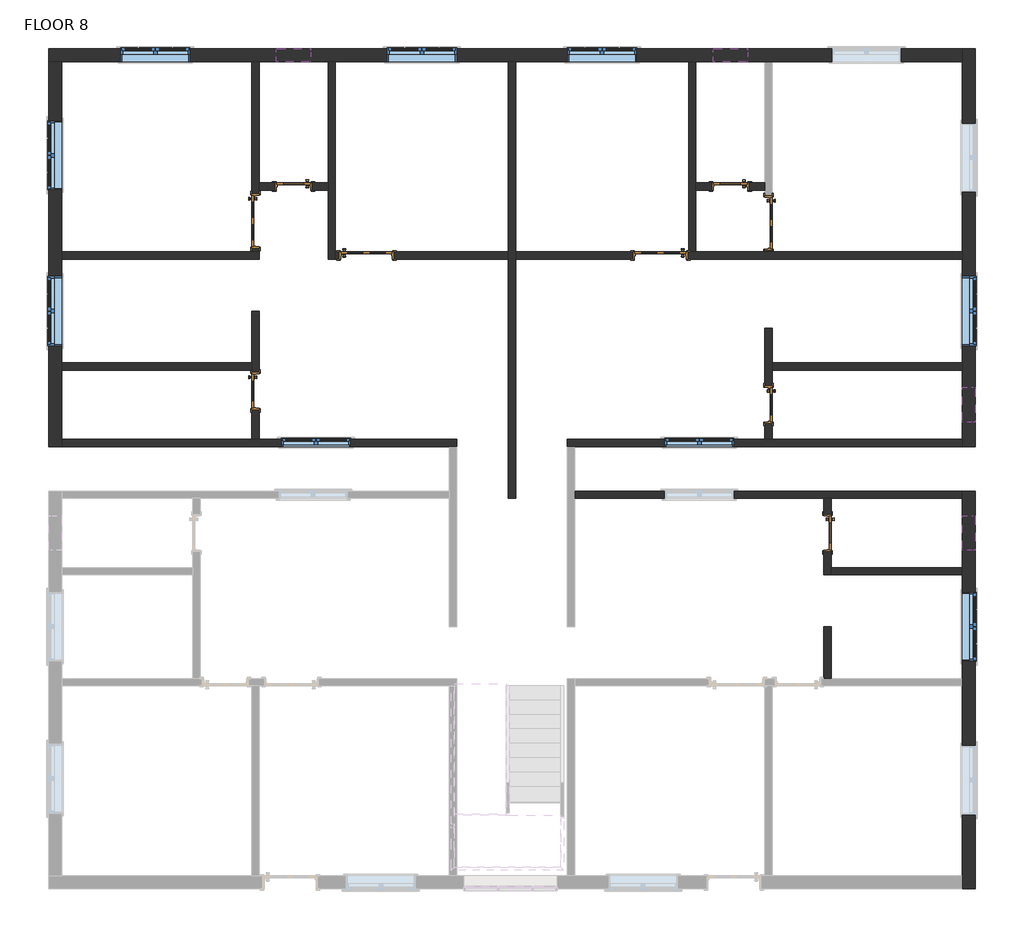
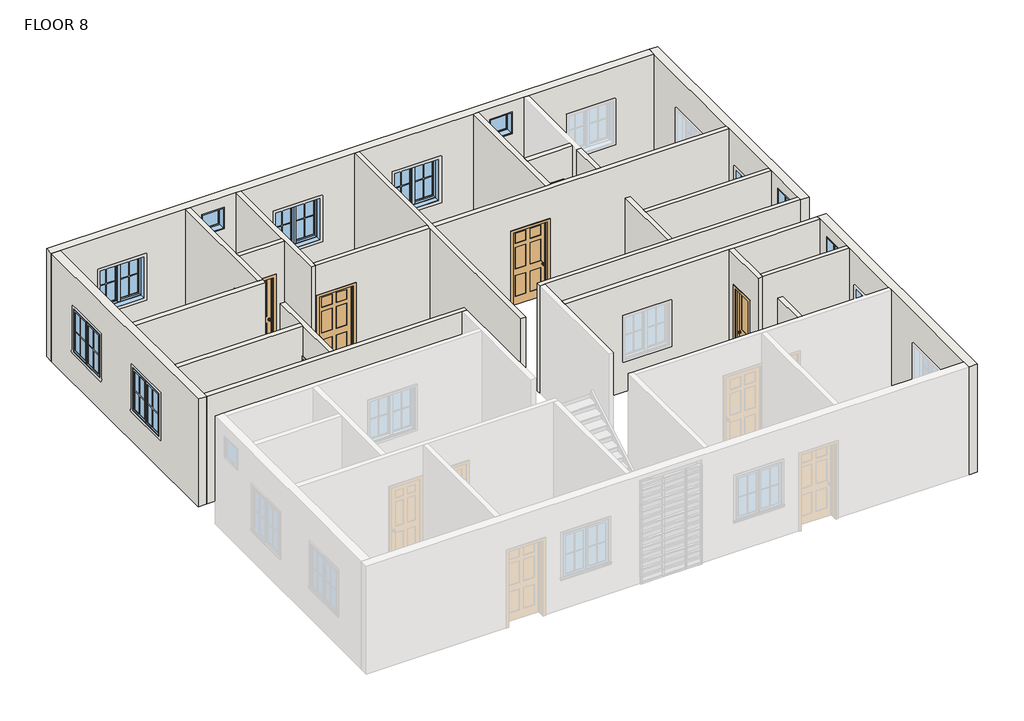
# One storey, part 3 of 4: 24 walls, 13 windows, 9 doors.
"""IFC4 building model written with IfcOpenShell, lengths in millimetres."""

from ifc_helpers import new_model, si_unit, frame, origin, place, context, project, spatial, polyline, outline, extrude, faceted_brep, transform, mapped, element, save
from components import door_e337afa5, door_596d7c92, door_c610b25b, door_03e3dfb5, window_80340324, window_9200f5ac, window_c2c97eee

model = new_model("IFC4")

# Units and contexts
model_context = context("Model", 3, world=origin())
ifc_project = project(units=[si_unit("LENGTHUNIT", "METRE", prefix="MILLI")], contexts=[model_context])

# Site, building, storey
site = spatial("IfcSite", under=ifc_project)
building = spatial("IfcBuilding", under=site)
storey = spatial("IfcBuildingStorey", under=building, Name="FLOOR 8", Elevation=12744.7725604)

# Doors
placement = place(None, origin())
door_shape = door_e337afa5(model_context)
element("IfcDoor", 1, ObjectType="Door-Interior-Single-2_Panel-Wood : 24\" x 84\"", at=placement, inside=storey, context=model_context, shape_type="MappedRepresentation", body=[
    mapped(door_shape, transform((-8112.4137331, 4563.2156164, 12744.7725604), x_axis=(-1.0, 0.0, 0.0), y_axis=(0.0, -1.0, 0.0), z_axis=(0.0, 0.0, 1.0))),
])
element("IfcDoor", 2, ObjectType="Door-Interior-Single-2_Panel-Wood : 24\" x 84\"", at=placement, inside=storey, context=model_context, shape_type="MappedRepresentation", body=[
    mapped(door_shape, transform((-416.2137331, 4563.2156164, 12744.7725604), x_axis=(-1.0, 0.0, 0.0), y_axis=(0.0, -1.0, 0.0), z_axis=(0.0, 0.0, 1.0))),
])
element("IfcDoor", 3, ObjectType="Door-Interior-Single-2_Panel-Wood : 24\" x 84\"", at=placement, inside=storey, context=model_context, shape_type="MappedRepresentation", body=[
    mapped(door_shape, transform((-8788.6887331, 953.2406164, 12744.7725604), x_axis=(0.0, -1.0, 0.0), y_axis=(1.0, 0.0, 0.0), z_axis=(0.0, 0.0, 1.0))),
])
door_2_shape = door_596d7c92(model_context)
element("IfcDoor", 4, ObjectType="Door-Interior-Single-2_Panel-Wood : 24\" x 84\"", at=placement, inside=storey, context=model_context, shape_type="MappedRepresentation", body=[
    mapped(door_2_shape, transform((260.0612669, 711.9406164, 12744.7725604), x_axis=(0.0, -1.0, 0.0), y_axis=(1.0, 0.0, 0.0), z_axis=(0.0, 0.0, 1.0))),
])
element("IfcDoor", 5, ObjectType="Door-Interior-Single-2_Panel-Wood : 24\" x 84\"", at=placement, inside=storey, context=model_context, shape_type="MappedRepresentation", body=[
    mapped(door_2_shape, transform((1301.4612669, -1548.6593836, 12744.7725604), x_axis=(0.0, -1.0, 0.0), y_axis=(1.0, 0.0, 0.0), z_axis=(0.0, 0.0, 1.0))),
])
door_3_shape = door_c610b25b(model_context)
element("IfcDoor", 6, ObjectType="Door-Interior-Single-6_Panel-Wood : 36\" x 84\"", at=placement, inside=storey, context=model_context, shape_type="MappedRepresentation", body=[
    mapped(door_3_shape, transform((-8788.6887331, 3950.4406164, 12744.7725604), x_axis=(0.0, -1.0, 0.0), y_axis=(1.0, 0.0, 0.0), z_axis=(0.0, 0.0, 1.0))),
])
element("IfcDoor", 7, ObjectType="Door-Interior-Single-6_Panel-Wood : 36\" x 84\"", at=placement, inside=storey, context=model_context, shape_type="MappedRepresentation", body=[
    mapped(door_3_shape, transform((-1648.1137331, 3344.0156164, 12744.7725604), x_axis=(-1.0, 0.0, 0.0), y_axis=(0.0, -1.0, 0.0), z_axis=(0.0, 0.0, 1.0))),
])
door_4_shape = door_03e3dfb5(model_context)
element("IfcDoor", 8, ObjectType="Door-Interior-Single-6_Panel-Wood : 36\" x 84\"", at=placement, inside=storey, context=model_context, shape_type="MappedRepresentation", body=[
    mapped(door_4_shape, transform((-6829.7137331, 3344.0156164, 12744.7725604), x_axis=(1.0, 0.0, 0.0), y_axis=(0.0, 1.0, 0.0), z_axis=(0.0, 0.0, 1.0))),
])
element("IfcDoor", 9, ObjectType="Door-Interior-Single-6_Panel-Wood : 36\" x 84\"", at=placement, inside=storey, context=model_context, shape_type="MappedRepresentation", body=[
    mapped(door_4_shape, transform((260.0612669, 3912.3406164, 12744.7725604), x_axis=(0.0, -1.0, 0.0), y_axis=(1.0, 0.0, 0.0), z_axis=(0.0, 0.0, 1.0))),
])

# Walls
element("IfcWall", 10, ObjectType="Inner Wall 5\"", at=placement, inside=storey, context=model_context, shape_type="Brep", body=[
    faceted_brep([(-12201.8137331, -24.6593836, 12744.7725604), (-5369.2137331, -24.6593836, 12744.7725604), (-5242.2137331, -24.6593836, 12744.7725604), (-5242.2137331, -24.6593836, 15792.7725604), (-5369.2137331, -24.6593836, 15792.7725604), (-12201.8137331, -24.6593836, 15792.7725604), (-7109.1137331, -24.6593836, 14878.3725604), (-7109.1137331, -24.6593836, 13659.1725604), (-8328.3137331, -24.6593836, 13659.1725604), (-8328.3137331, -24.6593836, 14878.3725604), (-12201.8137331, 102.3406164, 12744.7725604), (-12201.8137331, 102.3406164, 15792.7725604), (-8849.0137331, 102.3406164, 15792.7725604), (-8722.0137331, 102.3406164, 15792.7725604), (-5242.2137331, 102.3406164, 15792.7725604), (-5242.2137331, 102.3406164, 12744.7725604), (-8722.0137331, 102.3406164, 12744.7725604), (-8849.0137331, 102.3406164, 12744.7725604), (-7109.1137331, 102.3406164, 14878.3725604), (-8328.3137331, 102.3406164, 14878.3725604), (-8328.3137331, 102.3406164, 13659.1725604), (-7109.1137331, 102.3406164, 13659.1725604)], [[[0, 1, 2, 3, 4, 5], [6, 7, 8, 9]], [[10, 11, 12, 13, 14, 15, 16, 17], [18, 19, 20, 21]], [[2, 1, 0, 10, 17, 16, 15]], [[5, 4, 3, 14, 13, 12, 11]], [[0, 5, 11, 10]], [[3, 2, 15, 14]], [[7, 6, 18, 21]], [[8, 7, 21, 20]], [[9, 8, 20, 19]], [[6, 9, 19, 18]]]),
])
element("IfcWall", 11, ObjectType="Inner Wall 5\"", at=placement, inside=storey, context=model_context, shape_type="Brep", body=[
    faceted_brep([(3673.1862669, 102.3406164, 12744.7725604), (320.3862669, 102.3406164, 12744.7725604), (193.3862669, 102.3406164, 12744.7725604), (-3286.4137331, 102.3406164, 12744.7725604), (-3286.4137331, 102.3406164, 15792.7725604), (193.3862669, 102.3406164, 15792.7725604), (320.3862669, 102.3406164, 15792.7725604), (3673.1862669, 102.3406164, 15792.7725604), (-352.7137331, 102.3406164, 14878.3725604), (-1571.9137331, 102.3406164, 14878.3725604), (-1571.9137331, 102.3406164, 13659.1725604), (-352.7137331, 102.3406164, 13659.1725604), (3673.1862669, -24.6593836, 12744.7725604), (3673.1862669, -24.6593836, 15792.7725604), (-3159.4137331, -24.6593836, 15792.7725604), (-3286.4137331, -24.6593836, 15792.7725604), (-3286.4137331, -24.6593836, 12744.7725604), (-3159.4137331, -24.6593836, 12744.7725604), (-352.7137331, -24.6593836, 14878.3725604), (-352.7137331, -24.6593836, 13659.1725604), (-1571.9137331, -24.6593836, 13659.1725604), (-1571.9137331, -24.6593836, 14878.3725604)], [[[0, 1, 2, 3, 4, 5, 6, 7], [8, 9, 10, 11]], [[12, 13, 14, 15, 16, 17], [18, 19, 20, 21]], [[3, 2, 1, 0, 12, 17, 16]], [[7, 6, 5, 4, 15, 14, 13]], [[0, 7, 13, 12]], [[4, 3, 16, 15]], [[19, 18, 8, 11]], [[20, 19, 11, 10]], [[21, 20, 10, 9]], [[18, 21, 9, 8]]]),
])
element("IfcWall", 12, ObjectType="Inner Wall 5\"", at=placement, inside=storey, context=model_context, shape_type="Brep", body=[
    faceted_brep([(3673.1862669, -812.0593836, 12744.7725604), (-3159.4137331, -812.0593836, 12744.7725604), (-3159.4137331, -812.0593836, 15792.7725604), (3673.1862669, -812.0593836, 15792.7725604), (-352.7137331, -812.0593836, 14878.3725604), (-1571.9137331, -812.0593836, 14878.3725604), (-1571.9137331, -812.0593836, 13659.1725604), (-352.7137331, -812.0593836, 13659.1725604), (3673.1862669, -939.0593836, 12744.7725604), (3673.1862669, -939.0593836, 15792.7725604), (1361.7862669, -939.0593836, 15792.7725604), (1234.7862669, -939.0593836, 15792.7725604), (-3159.4137331, -939.0593836, 15792.7725604), (-3159.4137331, -939.0593836, 12744.7725604), (1234.7862669, -939.0593836, 12744.7725604), (1361.7862669, -939.0593836, 12744.7725604), (-352.7137331, -939.0593836, 14878.3725604), (-352.7137331, -939.0593836, 13659.1725604), (-1571.9137331, -939.0593836, 13659.1725604), (-1571.9137331, -939.0593836, 14878.3725604)], [[[0, 1, 2, 3], [4, 5, 6, 7]], [[8, 9, 10, 11, 12, 13, 14, 15], [16, 17, 18, 19]], [[1, 0, 8, 15, 14, 13]], [[3, 2, 12, 11, 10, 9]], [[0, 3, 9, 8]], [[2, 1, 13, 12]], [[17, 16, 4, 7]], [[18, 17, 7, 6]], [[19, 18, 6, 5]], [[16, 19, 5, 4]]]),
])
element("IfcWall", 13, ObjectType="Inner Wall 5\"", at=placement, inside=storey, context=model_context, shape_type="Brep", body=[
    faceted_brep([(1234.7862669, -2285.2593836, 15792.7725604), (1234.7862669, -939.0593836, 15792.7725604), (1234.7862669, -939.0593836, 12744.7725604), (1234.7862669, -1218.4593836, 12744.7725604), (1234.7862669, -1218.4593836, 14903.7725604), (1234.7862669, -1878.8593836, 14903.7725604), (1234.7862669, -1878.8593836, 12744.7725604), (1234.7862669, -2285.2593836, 12744.7725604), (1361.7862669, -939.0593836, 15792.7725604), (1361.7862669, -2158.2593836, 15792.7725604), (1361.7862669, -2285.2593836, 15792.7725604), (1361.7862669, -2285.2593836, 12744.7725604), (1361.7862669, -2158.2593836, 12744.7725604), (1361.7862669, -1878.8593836, 12744.7725604), (1361.7862669, -1878.8593836, 14903.7725604), (1361.7862669, -1218.4593836, 14903.7725604), (1361.7862669, -1218.4593836, 12744.7725604), (1361.7862669, -939.0593836, 12744.7725604)], [[[0, 1, 2, 3, 4, 5, 6, 7]], [[8, 9, 10, 11, 12, 13, 14, 15, 16, 17]], [[2, 17, 16, 3]], [[11, 7, 6, 13, 12]], [[1, 0, 10, 9, 8]], [[2, 1, 8, 17]], [[0, 7, 11, 10]], [[5, 14, 13, 6]], [[14, 5, 4, 15]], [[15, 4, 3, 16]]]),
])
element("IfcWall", 14, ObjectType="Inner Wall 5\"", at=placement, inside=storey, context=model_context, shape_type="SweptSolid", body=[
    extrude(outline(polyline([(3673.1862669, -2285.2593836), (1361.7862669, -2285.2593836), (1361.7862669, -2158.2593836), (3673.1862669, -2158.2593836), (3673.1862669, -2285.2593836)])), frame((0.0, 0.0, 12744.7725604), z_axis=(0.0, 0.0, 1.0), x_axis=(1.0, 0.0, 0.0)), (0.0, 0.0, 1.0), 3048.0),
])
element("IfcWall", 15, ObjectType="Inner Wall 5\"", at=placement, inside=storey, context=model_context, shape_type="SweptSolid", body=[
    extrude(outline(polyline([(1361.7862669, -3199.6593836), (1361.7862669, -4114.0593836), (1234.7862669, -4114.0593836), (1234.7862669, -3199.6593836), (1361.7862669, -3199.6593836)])), frame((0.0, 0.0, 12744.7725604), z_axis=(0.0, 0.0, 1.0), x_axis=(1.0, 0.0, 0.0)), (0.0, 0.0, 1.0), 3048.0),
])
element("IfcWall", 16, ObjectType="Inner Wall 5\"", at=placement, inside=storey, context=model_context, shape_type="Brep", body=[
    faceted_brep([(-12201.8137331, 3277.3406164, 12744.7725604), (-8722.0137331, 3277.3406164, 12744.7725604), (-8722.0137331, 3277.3406164, 15792.7725604), (-12201.8137331, 3277.3406164, 15792.7725604), (-12201.8137331, 3404.3406164, 12744.7725604), (-12201.8137331, 3404.3406164, 15792.7725604), (-8849.0137331, 3404.3406164, 15792.7725604), (-8722.0137331, 3404.3406164, 15792.7725604), (-8722.0137331, 3404.3406164, 12744.7725604), (-8849.0137331, 3404.3406164, 12744.7725604)], [[[0, 1, 2, 3]], [[4, 5, 6, 7, 8, 9]], [[1, 0, 4, 9, 8]], [[3, 2, 7, 6, 5]], [[0, 3, 5, 4]], [[2, 1, 8, 7]]]),
])
element("IfcWall", 17, ObjectType="Inner Wall 5\"", at=placement, inside=storey, context=model_context, shape_type="Brep", body=[
    faceted_brep([(-8722.0137331, 6758.7281164, 15792.7725604), (-8722.0137331, 4623.5406164, 15792.7725604), (-8722.0137331, 4496.5406164, 15792.7725604), (-8722.0137331, 3404.3406164, 15792.7725604), (-8722.0137331, 3404.3406164, 12744.7725604), (-8722.0137331, 3467.8406164, 12744.7725604), (-8722.0137331, 3467.8406164, 14903.7725604), (-8722.0137331, 4433.0406164, 14903.7725604), (-8722.0137331, 4433.0406164, 12744.7725604), (-8722.0137331, 4496.5406164, 12744.7725604), (-8722.0137331, 4623.5406164, 12744.7725604), (-8722.0137331, 6758.7281164, 12744.7725604), (-8849.0137331, 3404.3406164, 15792.7725604), (-8849.0137331, 6758.7281164, 15792.7725604), (-8849.0137331, 6758.7281164, 12744.7725604), (-8849.0137331, 4433.0406164, 12744.7725604), (-8849.0137331, 4433.0406164, 14903.7725604), (-8849.0137331, 3467.8406164, 14903.7725604), (-8849.0137331, 3467.8406164, 12744.7725604), (-8849.0137331, 3404.3406164, 12744.7725604)], [[[0, 1, 2, 3, 4, 5, 6, 7, 8, 9, 10, 11]], [[12, 13, 14, 15, 16, 17, 18, 19]], [[4, 19, 18, 5]], [[14, 11, 10, 9, 8, 15]], [[3, 2, 1, 0, 13, 12]], [[4, 3, 12, 19]], [[0, 11, 14, 13]], [[17, 6, 5, 18]], [[6, 17, 16, 7]], [[7, 16, 15, 8]]]),
])
element("IfcWall", 18, ObjectType="Inner Wall 5\"", at=placement, inside=storey, context=model_context, shape_type="SweptSolid", body=[
    extrude(outline(polyline([(15792.7725604, -7502.8137331), (15792.7725604, -8722.0137331), (12744.7725604, -8722.0137331), (12744.7725604, -8442.6137331), (14903.7725604, -8442.6137331), (14903.7725604, -7782.2137331), (12744.7725604, -7782.2137331), (12744.7725604, -7502.8137331), (15792.7725604, -7502.8137331)])), frame((0.0, 4496.5406164, 0.0), z_axis=(0.0, 1.0, 0.0), x_axis=(0.0, 0.0, 1.0)), (0.0, 0.0, 1.0), 127.0),
])
element("IfcWall", 19, ObjectType="Inner Wall 5\"", at=placement, inside=storey, context=model_context, shape_type="Brep", body=[
    faceted_brep([(-7375.8137331, 3277.3406164, 12744.7725604), (-7375.8137331, 3404.3406164, 12744.7725604), (-7375.8137331, 6758.7281164, 12744.7725604), (-7375.8137331, 6758.7281164, 15792.7725604), (-7375.8137331, 3404.3406164, 15792.7725604), (-7375.8137331, 3277.3406164, 15792.7725604), (-7502.8137331, 3277.3406164, 12744.7725604), (-7502.8137331, 3277.3406164, 15792.7725604), (-7502.8137331, 4496.5406164, 15792.7725604), (-7502.8137331, 4623.5406164, 15792.7725604), (-7502.8137331, 6758.7281164, 15792.7725604), (-7502.8137331, 6758.7281164, 12744.7725604), (-7502.8137331, 4623.5406164, 12744.7725604), (-7502.8137331, 4496.5406164, 12744.7725604)], [[[0, 1, 2, 3, 4, 5]], [[6, 7, 8, 9, 10, 11, 12, 13]], [[2, 1, 0, 6, 13, 12, 11]], [[5, 4, 3, 10, 9, 8, 7]], [[3, 2, 11, 10]], [[0, 5, 7, 6]]]),
])
element("IfcWall", 20, ObjectType="Inner Wall 5\"", at=placement, inside=storey, context=model_context, shape_type="Brep", body=[
    faceted_brep([(-4327.8137331, 6758.7281164, 12744.7725604), (-4327.8137331, 3404.3406164, 12744.7725604), (-4327.8137331, 3277.3406164, 12744.7725604), (-4327.8137331, -939.0593836, 12744.7725604), (-4327.8137331, -939.0593836, 15792.7725604), (-4327.8137331, 3277.3406164, 15792.7725604), (-4327.8137331, 3404.3406164, 15792.7725604), (-4327.8137331, 6758.7281164, 15792.7725604), (-4200.8137331, 6758.7281164, 12744.7725604), (-4200.8137331, 6758.7281164, 15792.7725604), (-4200.8137331, 3404.3406164, 15792.7725604), (-4200.8137331, 3277.3406164, 15792.7725604), (-4200.8137331, -939.0593836, 15792.7725604), (-4200.8137331, -939.0593836, 12744.7725604), (-4200.8137331, 3277.3406164, 12744.7725604), (-4200.8137331, 3404.3406164, 12744.7725604)], [[[0, 1, 2, 3, 4, 5, 6, 7]], [[8, 9, 10, 11, 12, 13, 14, 15]], [[3, 2, 1, 0, 8, 15, 14, 13]], [[4, 3, 13, 12]], [[7, 6, 5, 4, 12, 11, 10, 9]], [[0, 7, 9, 8]]]),
])
element("IfcWall", 21, ObjectType="Inner Wall 5\"", at=placement, inside=storey, context=model_context, shape_type="SweptSolid", body=[
    extrude(outline(polyline([(15792.7725604, -4327.8137331), (15792.7725604, -7375.8137331), (12744.7725604, -7375.8137331), (12744.7725604, -7312.3137331), (14903.7725604, -7312.3137331), (14903.7725604, -6347.1137331), (12744.7725604, -6347.1137331), (12744.7725604, -4327.8137331), (15792.7725604, -4327.8137331)])), frame((0.0, 3277.3406164, 0.0), z_axis=(0.0, 1.0, 0.0), x_axis=(0.0, 0.0, 1.0)), (0.0, 0.0, 1.0), 127.0),
])
element("IfcWall", 22, ObjectType="Inner Wall 5\"", at=placement, inside=storey, context=model_context, shape_type="Brep", body=[
    faceted_brep([(3673.1862669, 3277.3406164, 15792.7725604), (-4200.8137331, 3277.3406164, 15792.7725604), (-4200.8137331, 3277.3406164, 12744.7725604), (-2130.7137331, 3277.3406164, 12744.7725604), (-2130.7137331, 3277.3406164, 14903.7725604), (-1165.5137331, 3277.3406164, 14903.7725604), (-1165.5137331, 3277.3406164, 12744.7725604), (3673.1862669, 3277.3406164, 12744.7725604), (-4200.8137331, 3404.3406164, 15792.7725604), (-1152.8137331, 3404.3406164, 15792.7725604), (-1025.8137331, 3404.3406164, 15792.7725604), (193.3862669, 3404.3406164, 15792.7725604), (320.3862669, 3404.3406164, 15792.7725604), (3673.1862669, 3404.3406164, 15792.7725604), (3673.1862669, 3404.3406164, 12744.7725604), (320.3862669, 3404.3406164, 12744.7725604), (193.3862669, 3404.3406164, 12744.7725604), (-1025.8137331, 3404.3406164, 12744.7725604), (-1152.8137331, 3404.3406164, 12744.7725604), (-1165.5137331, 3404.3406164, 12744.7725604), (-1165.5137331, 3404.3406164, 14903.7725604), (-2130.7137331, 3404.3406164, 14903.7725604), (-2130.7137331, 3404.3406164, 12744.7725604), (-4200.8137331, 3404.3406164, 12744.7725604)], [[[0, 1, 2, 3, 4, 5, 6, 7]], [[8, 9, 10, 11, 12, 13, 14, 15, 16, 17, 18, 19, 20, 21, 22, 23]], [[2, 23, 22, 3]], [[14, 7, 6, 19, 18, 17, 16, 15]], [[1, 0, 13, 12, 11, 10, 9, 8]], [[2, 1, 8, 23]], [[0, 7, 14, 13]], [[21, 4, 3, 22]], [[4, 21, 20, 5]], [[5, 20, 19, 6]]]),
])
element("IfcWall", 23, ObjectType="Inner Wall 5\"", at=placement, inside=storey, context=model_context, shape_type="Brep", body=[
    faceted_brep([(-1025.8137331, 3404.3406164, 12744.7725604), (-1025.8137331, 4496.5406164, 12744.7725604), (-1025.8137331, 4623.5406164, 12744.7725604), (-1025.8137331, 6758.7281164, 12744.7725604), (-1025.8137331, 6758.7281164, 15792.7725604), (-1025.8137331, 4623.5406164, 15792.7725604), (-1025.8137331, 4496.5406164, 15792.7725604), (-1025.8137331, 3404.3406164, 15792.7725604), (-1152.8137331, 3404.3406164, 12744.7725604), (-1152.8137331, 3404.3406164, 15792.7725604), (-1152.8137331, 6758.7281164, 15792.7725604), (-1152.8137331, 6758.7281164, 12744.7725604)], [[[0, 1, 2, 3, 4, 5, 6, 7]], [[8, 9, 10, 11]], [[3, 2, 1, 0, 8, 11]], [[7, 6, 5, 4, 10, 9]], [[0, 7, 9, 8]], [[4, 3, 11, 10]]]),
])
element("IfcWall", 24, ObjectType="Inner Wall 5\"", at=placement, inside=storey, context=model_context, shape_type="SweptSolid", body=[
    extrude(outline(polyline([(15792.7725604, 193.3862669), (15792.7725604, -1025.8137331), (12744.7725604, -1025.8137331), (12744.7725604, -746.4137331), (14903.7725604, -746.4137331), (14903.7725604, -86.0137331), (12744.7725604, -86.0137331), (12744.7725604, 193.3862669), (15792.7725604, 193.3862669)])), frame((0.0, 4496.5406164, 0.0), z_axis=(0.0, 1.0, 0.0), x_axis=(0.0, 0.0, 1.0)), (0.0, 0.0, 1.0), 127.0),
])
element("IfcWall", 25, ObjectType="Inner Wall 5\"", at=placement, inside=storey, context=model_context, shape_type="SweptSolid", body=[
    extrude(outline(polyline([(320.3862669, 1448.5406164), (3673.1862669, 1448.5406164), (3673.1862669, 1321.5406164), (320.3862669, 1321.5406164), (320.3862669, 1448.5406164)])), frame((0.0, 0.0, 12744.7725604), z_axis=(0.0, 0.0, 1.0), x_axis=(1.0, 0.0, 0.0)), (0.0, 0.0, 1.0), 3048.0),
])
element("IfcWall", 26, ObjectType="Inner Wall 5\"", at=placement, inside=storey, context=model_context, shape_type="Brep", body=[
    faceted_brep([(193.3862669, 102.3406164, 15792.7725604), (193.3862669, 2058.1406164, 15792.7725604), (193.3862669, 2058.1406164, 12744.7725604), (193.3862669, 1042.1406164, 12744.7725604), (193.3862669, 1042.1406164, 14903.7725604), (193.3862669, 381.7406164, 14903.7725604), (193.3862669, 381.7406164, 12744.7725604), (193.3862669, 102.3406164, 12744.7725604), (320.3862669, 2058.1406164, 15792.7725604), (320.3862669, 1448.5406164, 15792.7725604), (320.3862669, 1321.5406164, 15792.7725604), (320.3862669, 102.3406164, 15792.7725604), (320.3862669, 102.3406164, 12744.7725604), (320.3862669, 381.7406164, 12744.7725604), (320.3862669, 381.7406164, 14903.7725604), (320.3862669, 1042.1406164, 14903.7725604), (320.3862669, 1042.1406164, 12744.7725604), (320.3862669, 1321.5406164, 12744.7725604), (320.3862669, 1448.5406164, 12744.7725604), (320.3862669, 2058.1406164, 12744.7725604)], [[[0, 1, 2, 3, 4, 5, 6, 7]], [[8, 9, 10, 11, 12, 13, 14, 15, 16, 17, 18, 19]], [[2, 19, 18, 17, 16, 3]], [[12, 7, 6, 13]], [[1, 0, 11, 10, 9, 8]], [[2, 1, 8, 19]], [[0, 7, 12, 11]], [[5, 14, 13, 6]], [[14, 5, 4, 15]], [[15, 4, 3, 16]]]),
])
element("IfcWall", 27, ObjectType="Inner Wall 5\"", at=placement, inside=storey, context=model_context, shape_type="Brep", body=[
    faceted_brep([(-8722.0137331, 2362.9406164, 12744.7725604), (-8722.0137331, 2362.9406164, 15792.7725604), (-8722.0137331, 102.3406164, 15792.7725604), (-8722.0137331, 102.3406164, 12744.7725604), (-8722.0137331, 623.0406164, 12744.7725604), (-8722.0137331, 623.0406164, 14903.7725604), (-8722.0137331, 1283.4406164, 14903.7725604), (-8722.0137331, 1283.4406164, 12744.7725604), (-8849.0137331, 2362.9406164, 15792.7725604), (-8849.0137331, 2362.9406164, 12744.7725604), (-8849.0137331, 1448.5406164, 12744.7725604), (-8849.0137331, 1321.5406164, 12744.7725604), (-8849.0137331, 1283.4406164, 12744.7725604), (-8849.0137331, 1283.4406164, 14903.7725604), (-8849.0137331, 623.0406164, 14903.7725604), (-8849.0137331, 623.0406164, 12744.7725604), (-8849.0137331, 102.3406164, 12744.7725604), (-8849.0137331, 102.3406164, 15792.7725604), (-8849.0137331, 1321.5406164, 15792.7725604), (-8849.0137331, 1448.5406164, 15792.7725604)], [[[0, 1, 2, 3, 4, 5, 6, 7]], [[8, 9, 10, 11, 12, 13, 14, 15, 16, 17, 18, 19]], [[9, 0, 7, 12, 11, 10]], [[3, 16, 15, 4]], [[1, 0, 9, 8]], [[2, 1, 8, 19, 18, 17]], [[3, 2, 17, 16]], [[14, 5, 4, 15]], [[5, 14, 13, 6]], [[6, 13, 12, 7]]]),
])
element("IfcWall", 28, ObjectType="Inner Wall 5\"", at=placement, inside=storey, context=model_context, shape_type="SweptSolid", body=[
    extrude(outline(polyline([(-12201.8137331, 1448.5406164), (-8849.0137331, 1448.5406164), (-8849.0137331, 1321.5406164), (-12201.8137331, 1321.5406164), (-12201.8137331, 1448.5406164)])), frame((0.0, 0.0, 12744.7725604), z_axis=(0.0, 0.0, 1.0), x_axis=(1.0, 0.0, 0.0)), (0.0, 0.0, 1.0), 3048.0),
])
element("IfcWall", 29, ObjectType="Inner Wall 5\"", at=placement, inside=storey, context=model_context, shape_type="SweptSolid", body=[
    extrude(outline(polyline([(3404.3406164, 15792.7725604), (4318.7406164, 15792.7725604), (4318.7406164, 14903.7725604), (3429.7406164, 14903.7725604), (3429.7406164, 12744.7725604), (3404.3406164, 12744.7725604), (3404.3406164, 15792.7725604)])), frame((193.3862669, 0.0, 0.0), z_axis=(1.0, 0.0, 0.0), x_axis=(0.0, 1.0, 0.0)), (0.0, 0.0, 1.0), 127.0),
])
element("IfcWall", 30, ObjectType="outer wall 9\"", at=placement, inside=storey, context=model_context, shape_type="Brep", body=[
    faceted_brep([(-12430.4137331, 6758.7281164, 12744.7725604), (-12201.8137331, 6758.7281164, 12744.7725604), (-8849.0137331, 6758.7281164, 12744.7725604), (-8722.0137331, 6758.7281164, 12744.7725604), (-7502.8137331, 6758.7281164, 12744.7725604), (-7375.8137331, 6758.7281164, 12744.7725604), (-4327.8137331, 6758.7281164, 12744.7725604), (-4200.8137331, 6758.7281164, 12744.7725604), (-1152.8137331, 6758.7281164, 12744.7725604), (-1025.8137331, 6758.7281164, 12744.7725604), (193.3862669, 6758.7281164, 12744.7725604), (320.3862669, 6758.7281164, 12744.7725604), (3673.1862669, 6758.7281164, 12744.7725604), (3673.1862669, 6758.7281164, 15792.7725604), (320.3862669, 6758.7281164, 15792.7725604), (193.3862669, 6758.7281164, 15792.7725604), (-1025.8137331, 6758.7281164, 15792.7725604), (-1152.8137331, 6758.7281164, 15792.7725604), (-4200.8137331, 6758.7281164, 15792.7725604), (-4327.8137331, 6758.7281164, 15792.7725604), (-7375.8137331, 6758.7281164, 15792.7725604), (-7502.8137331, 6758.7281164, 15792.7725604), (-8722.0137331, 6758.7281164, 15792.7725604), (-8849.0137331, 6758.7281164, 15792.7725604), (-12201.8137331, 6758.7281164, 15792.7725604), (-12430.4137331, 6758.7281164, 15792.7725604), (-9941.2137331, 6758.7281164, 14878.3725604), (-9941.2137331, 6758.7281164, 13659.1725604), (-11160.4137331, 6758.7281164, 13659.1725604), (-11160.4137331, 6758.7281164, 14878.3725604), (-5242.2137331, 6758.7281164, 14878.3725604), (-5242.2137331, 6758.7281164, 13659.1725604), (-6461.4137331, 6758.7281164, 13659.1725604), (-6461.4137331, 6758.7281164, 14878.3725604), (-2067.2137331, 6758.7281164, 14878.3725604), (-2067.2137331, 6758.7281164, 13659.1725604), (-3286.4137331, 6758.7281164, 13659.1725604), (-3286.4137331, 6758.7281164, 14878.3725604), (2593.6862669, 6758.7281164, 14878.3725604), (2593.6862669, 6758.7281164, 13659.1725604), (1374.4862669, 6758.7281164, 13659.1725604), (1374.4862669, 6758.7281164, 14878.3725604), (-7807.6137331, 6758.7281164, 15487.9725604), (-7807.6137331, 6758.7281164, 14878.3725604), (-8417.2137331, 6758.7281164, 14878.3725604), (-8417.2137331, 6758.7281164, 15487.9725604), (-111.4137331, 6758.7281164, 15487.9725604), (-111.4137331, 6758.7281164, 14878.3725604), (-721.0137331, 6758.7281164, 14878.3725604), (-721.0137331, 6758.7281164, 15487.9725604), (-12430.4137331, 6987.3281164, 12744.7725604), (-12430.4137331, 6987.3281164, 15792.7725604), (3673.1862669, 6987.3281164, 15792.7725604), (3673.1862669, 6987.3281164, 12744.7725604), (-9941.2137331, 6987.3281164, 14878.3725604), (-11160.4137331, 6987.3281164, 14878.3725604), (-11160.4137331, 6987.3281164, 13659.1725604), (-9941.2137331, 6987.3281164, 13659.1725604), (-5242.2137331, 6987.3281164, 14878.3725604), (-6461.4137331, 6987.3281164, 14878.3725604), (-6461.4137331, 6987.3281164, 13659.1725604), (-5242.2137331, 6987.3281164, 13659.1725604), (-2067.2137331, 6987.3281164, 14878.3725604), (-3286.4137331, 6987.3281164, 14878.3725604), (-3286.4137331, 6987.3281164, 13659.1725604), (-2067.2137331, 6987.3281164, 13659.1725604), (2593.6862669, 6987.3281164, 14878.3725604), (1374.4862669, 6987.3281164, 14878.3725604), (1374.4862669, 6987.3281164, 13659.1725604), (2593.6862669, 6987.3281164, 13659.1725604), (-7807.6137331, 6987.3281164, 15487.9725604), (-8417.2137331, 6987.3281164, 15487.9725604), (-8417.2137331, 6987.3281164, 14878.3725604), (-7807.6137331, 6987.3281164, 14878.3725604), (-111.4137331, 6987.3281164, 15487.9725604), (-721.0137331, 6987.3281164, 15487.9725604), (-721.0137331, 6987.3281164, 14878.3725604), (-111.4137331, 6987.3281164, 14878.3725604)], [[[0, 1, 2, 3, 4, 5, 6, 7, 8, 9, 10, 11, 12, 13, 14, 15, 16, 17, 18, 19, 20, 21, 22, 23, 24, 25], [26, 27, 28, 29], [30, 31, 32, 33], [34, 35, 36, 37], [38, 39, 40, 41], [42, 43, 44, 45], [46, 47, 48, 49]], [[50, 51, 52, 53], [54, 55, 56, 57], [58, 59, 60, 61], [62, 63, 64, 65], [66, 67, 68, 69], [70, 71, 72, 73], [74, 75, 76, 77]], [[12, 11, 10, 9, 8, 7, 6, 5, 4, 3, 2, 1, 0, 50, 53]], [[25, 24, 23, 22, 21, 20, 19, 18, 17, 16, 15, 14, 13, 52, 51]], [[0, 25, 51, 50]], [[13, 12, 53, 52]], [[27, 26, 54, 57]], [[28, 27, 57, 56]], [[29, 28, 56, 55]], [[26, 29, 55, 54]], [[31, 30, 58, 61]], [[32, 31, 61, 60]], [[33, 32, 60, 59]], [[30, 33, 59, 58]], [[35, 34, 62, 65]], [[36, 35, 65, 64]], [[37, 36, 64, 63]], [[34, 37, 63, 62]], [[39, 38, 66, 69]], [[40, 39, 69, 68]], [[41, 40, 68, 67]], [[38, 41, 67, 66]], [[43, 42, 70, 73]], [[44, 43, 73, 72]], [[45, 44, 72, 71]], [[42, 45, 71, 70]], [[47, 46, 74, 77]], [[48, 47, 77, 76]], [[49, 48, 76, 75]], [[46, 49, 75, 74]]]),
])
element("IfcWall", 31, ObjectType="outer wall 9\"", at=placement, inside=storey, context=model_context, shape_type="Brep", body=[
    faceted_brep([(-12201.8137331, -24.6593836, 12744.7725604), (-12201.8137331, 102.3406164, 12744.7725604), (-12201.8137331, 1321.5406164, 12744.7725604), (-12201.8137331, 1448.5406164, 12744.7725604), (-12201.8137331, 3277.3406164, 12744.7725604), (-12201.8137331, 3404.3406164, 12744.7725604), (-12201.8137331, 6758.7281164, 12744.7725604), (-12201.8137331, 6758.7281164, 15792.7725604), (-12201.8137331, 3404.3406164, 15792.7725604), (-12201.8137331, 3277.3406164, 15792.7725604), (-12201.8137331, 1448.5406164, 15792.7725604), (-12201.8137331, 1321.5406164, 15792.7725604), (-12201.8137331, 102.3406164, 15792.7725604), (-12201.8137331, -24.6593836, 15792.7725604), (-12201.8137331, 2972.5406164, 14878.3725604), (-12201.8137331, 2972.5406164, 13659.1725604), (-12201.8137331, 1753.3406164, 13659.1725604), (-12201.8137331, 1753.3406164, 14878.3725604), (-12201.8137331, 5716.5343664, 14878.3725604), (-12201.8137331, 5716.5343664, 13659.1725604), (-12201.8137331, 4497.3343664, 13659.1725604), (-12201.8137331, 4497.3343664, 14878.3725604), (-12430.4137331, -24.6593836, 12744.7725604), (-12430.4137331, -24.6593836, 15792.7725604), (-12430.4137331, 6758.7281164, 15792.7725604), (-12430.4137331, 6758.7281164, 12744.7725604), (-12430.4137331, 2972.5406164, 14878.3725604), (-12430.4137331, 1753.3406164, 14878.3725604), (-12430.4137331, 1753.3406164, 13659.1725604), (-12430.4137331, 2972.5406164, 13659.1725604), (-12430.4137331, 5716.5343664, 14878.3725604), (-12430.4137331, 4497.3343664, 14878.3725604), (-12430.4137331, 4497.3343664, 13659.1725604), (-12430.4137331, 5716.5343664, 13659.1725604)], [[[0, 1, 2, 3, 4, 5, 6, 7, 8, 9, 10, 11, 12, 13], [14, 15, 16, 17], [18, 19, 20, 21]], [[22, 23, 24, 25], [26, 27, 28, 29], [30, 31, 32, 33]], [[6, 5, 4, 3, 2, 1, 0, 22, 25]], [[13, 12, 11, 10, 9, 8, 7, 24, 23]], [[7, 6, 25, 24]], [[0, 13, 23, 22]], [[15, 14, 26, 29]], [[16, 15, 29, 28]], [[17, 16, 28, 27]], [[14, 17, 27, 26]], [[19, 18, 30, 33]], [[20, 19, 33, 32]], [[21, 20, 32, 31]], [[18, 21, 31, 30]]]),
])
element("IfcWall", 32, ObjectType="outer wall 9\"", at=placement, inside=storey, context=model_context, shape_type="Brep", body=[
    faceted_brep([(3673.1862669, 6987.3281164, 12744.7725604), (3673.1862669, 6758.7281164, 12744.7725604), (3673.1862669, 3404.3406164, 12744.7725604), (3673.1862669, 3277.3406164, 12744.7725604), (3673.1862669, 1448.5406164, 12744.7725604), (3673.1862669, 1321.5406164, 12744.7725604), (3673.1862669, 102.3406164, 12744.7725604), (3673.1862669, -24.6593836, 12744.7725604), (3673.1862669, -24.6593836, 15792.7725604), (3673.1862669, 102.3406164, 15792.7725604), (3673.1862669, 1321.5406164, 15792.7725604), (3673.1862669, 1448.5406164, 15792.7725604), (3673.1862669, 3277.3406164, 15792.7725604), (3673.1862669, 3404.3406164, 15792.7725604), (3673.1862669, 6758.7281164, 15792.7725604), (3673.1862669, 6987.3281164, 15792.7725604), (3673.1862669, 4458.4406164, 14878.3725604), (3673.1862669, 4458.4406164, 13659.1725604), (3673.1862669, 5677.6406164, 13659.1725604), (3673.1862669, 5677.6406164, 14878.3725604), (3673.1862669, 1753.3406164, 14878.3725604), (3673.1862669, 1753.3406164, 13659.1725604), (3673.1862669, 2972.5406164, 13659.1725604), (3673.1862669, 2972.5406164, 14878.3725604), (3673.1862669, 407.1406164, 15487.9725604), (3673.1862669, 407.1406164, 14878.3725604), (3673.1862669, 1016.7406164, 14878.3725604), (3673.1862669, 1016.7406164, 15487.9725604), (3901.7862669, 6987.3281164, 12744.7725604), (3901.7862669, 6987.3281164, 15792.7725604), (3901.7862669, -24.6593836, 15792.7725604), (3901.7862669, -24.6593836, 12744.7725604), (3901.7862669, 4458.4406164, 14878.3725604), (3901.7862669, 5677.6406164, 14878.3725604), (3901.7862669, 5677.6406164, 13659.1725604), (3901.7862669, 4458.4406164, 13659.1725604), (3901.7862669, 1753.3406164, 14878.3725604), (3901.7862669, 2972.5406164, 14878.3725604), (3901.7862669, 2972.5406164, 13659.1725604), (3901.7862669, 1753.3406164, 13659.1725604), (3901.7862669, 407.1406164, 15487.9725604), (3901.7862669, 1016.7406164, 15487.9725604), (3901.7862669, 1016.7406164, 14878.3725604), (3901.7862669, 407.1406164, 14878.3725604)], [[[0, 1, 2, 3, 4, 5, 6, 7, 8, 9, 10, 11, 12, 13, 14, 15], [16, 17, 18, 19], [20, 21, 22, 23], [24, 25, 26, 27]], [[28, 29, 30, 31], [32, 33, 34, 35], [36, 37, 38, 39], [40, 41, 42, 43]], [[7, 6, 5, 4, 3, 2, 1, 0, 28, 31]], [[15, 14, 13, 12, 11, 10, 9, 8, 30, 29]], [[0, 15, 29, 28]], [[8, 7, 31, 30]], [[17, 16, 32, 35]], [[18, 17, 35, 34]], [[19, 18, 34, 33]], [[16, 19, 33, 32]], [[21, 20, 36, 39]], [[22, 21, 39, 38]], [[23, 22, 38, 37]], [[20, 23, 37, 36]], [[25, 24, 40, 43]], [[26, 25, 43, 42]], [[27, 26, 42, 41]], [[24, 27, 41, 40]]]),
])
element("IfcWall", 33, ObjectType="outer wall 9\"", at=placement, inside=storey, context=model_context, shape_type="Brep", body=[
    faceted_brep([(3901.7862669, -7822.4593836, 12744.7725604), (3901.7862669, -812.0593836, 12744.7725604), (3901.7862669, -812.0593836, 15792.7725604), (3901.7862669, -7822.4593836, 15792.7725604), (3901.7862669, -3809.2593836, 14878.3725604), (3901.7862669, -2590.0593836, 14878.3725604), (3901.7862669, -2590.0593836, 13659.1725604), (3901.7862669, -3809.2593836, 13659.1725604), (3901.7862669, -6514.3593836, 14878.3725604), (3901.7862669, -5295.1593836, 14878.3725604), (3901.7862669, -5295.1593836, 13659.1725604), (3901.7862669, -6514.3593836, 13659.1725604), (3901.7862669, -1853.4593836, 15487.9725604), (3901.7862669, -1243.8593836, 15487.9725604), (3901.7862669, -1243.8593836, 14878.3725604), (3901.7862669, -1853.4593836, 14878.3725604), (3673.1862669, -7822.4593836, 12744.7725604), (3673.1862669, -7822.4593836, 15792.7725604), (3673.1862669, -7593.8593836, 15792.7725604), (3673.1862669, -4241.0593836, 15792.7725604), (3673.1862669, -4114.0593836, 15792.7725604), (3673.1862669, -2285.2593836, 15792.7725604), (3673.1862669, -2158.2593836, 15792.7725604), (3673.1862669, -939.0593836, 15792.7725604), (3673.1862669, -812.0593836, 15792.7725604), (3673.1862669, -812.0593836, 12744.7725604), (3673.1862669, -939.0593836, 12744.7725604), (3673.1862669, -2158.2593836, 12744.7725604), (3673.1862669, -2285.2593836, 12744.7725604), (3673.1862669, -4114.0593836, 12744.7725604), (3673.1862669, -4241.0593836, 12744.7725604), (3673.1862669, -7593.8593836, 12744.7725604), (3673.1862669, -3809.2593836, 14878.3725604), (3673.1862669, -3809.2593836, 13659.1725604), (3673.1862669, -2590.0593836, 13659.1725604), (3673.1862669, -2590.0593836, 14878.3725604), (3673.1862669, -6514.3593836, 14878.3725604), (3673.1862669, -6514.3593836, 13659.1725604), (3673.1862669, -5295.1593836, 13659.1725604), (3673.1862669, -5295.1593836, 14878.3725604), (3673.1862669, -1853.4593836, 15487.9725604), (3673.1862669, -1853.4593836, 14878.3725604), (3673.1862669, -1243.8593836, 14878.3725604), (3673.1862669, -1243.8593836, 15487.9725604)], [[[0, 1, 2, 3], [4, 5, 6, 7], [8, 9, 10, 11], [12, 13, 14, 15]], [[16, 17, 18, 19, 20, 21, 22, 23, 24, 25, 26, 27, 28, 29, 30, 31], [32, 33, 34, 35], [36, 37, 38, 39], [40, 41, 42, 43]], [[1, 0, 16, 31, 30, 29, 28, 27, 26, 25]], [[3, 2, 24, 23, 22, 21, 20, 19, 18, 17]], [[0, 3, 17, 16]], [[2, 1, 25, 24]], [[33, 32, 4, 7]], [[34, 33, 7, 6]], [[35, 34, 6, 5]], [[32, 35, 5, 4]], [[37, 36, 8, 11]], [[38, 37, 11, 10]], [[39, 38, 10, 9]], [[36, 39, 9, 8]], [[41, 40, 12, 15]], [[42, 41, 15, 14]], [[43, 42, 14, 13]], [[40, 43, 13, 12]]]),
])

# Windows
window_shape = window_80340324(model_context)
element("IfcWindow", 34, ObjectType="Fixed : 24\" x 24\"", at=placement, inside=storey, context=model_context, shape_type="MappedRepresentation", body=[
    mapped(window_shape, transform((3787.4862669, -1586.7593836, 13963.9725604), x_axis=(0.0, -1.0, 0.0), y_axis=(1.0, 0.0, 0.0), z_axis=(0.0, 0.0, 1.0))),
])
element("IfcWindow", 35, ObjectType="Fixed : 24\" x 24\"", at=placement, inside=storey, context=model_context, shape_type="MappedRepresentation", body=[
    mapped(window_shape, transform((3787.4862669, 673.8406164, 13963.9725604), x_axis=(0.0, -1.0, 0.0), y_axis=(1.0, 0.0, 0.0), z_axis=(0.0, 0.0, 1.0))),
])
element("IfcWindow", 36, ObjectType="Fixed : 24\" x 24\"", at=placement, inside=storey, context=model_context, shape_type="MappedRepresentation", body=[
    mapped(window_shape, transform((-8074.3137331, 6873.0281164, 13963.9725604), x_axis=(1.0, 0.0, 0.0), y_axis=(0.0, 1.0, 0.0), z_axis=(0.0, 0.0, 1.0))),
])
element("IfcWindow", 37, ObjectType="Fixed : 24\" x 24\"", at=placement, inside=storey, context=model_context, shape_type="MappedRepresentation", body=[
    mapped(window_shape, transform((-378.1137331, 6873.0281164, 13963.9725604), x_axis=(1.0, 0.0, 0.0), y_axis=(0.0, 1.0, 0.0), z_axis=(0.0, 0.0, 1.0))),
])
window_2_shape = window_9200f5ac(model_context)
element("IfcWindow", 38, ObjectType="Window-Casement-Double : 48\" x 48\"", at=placement, inside=storey, context=model_context, shape_type="MappedRepresentation", body=[
    mapped(window_2_shape, transform((-12316.1137331, 2362.9406164, 12744.7725604), x_axis=(0.0, 1.0, 0.0), y_axis=(-1.0, 0.0, 0.0), z_axis=(0.0, 0.0, 1.0))),
])
element("IfcWindow", 39, ObjectType="Window-Casement-Double : 48\" x 48\"", at=placement, inside=storey, context=model_context, shape_type="MappedRepresentation", body=[
    mapped(window_2_shape, transform((-12316.1137331, 5106.9343664, 12744.7725604), x_axis=(0.0, 1.0, 0.0), y_axis=(-1.0, 0.0, 0.0), z_axis=(0.0, 0.0, 1.0))),
])
element("IfcWindow", 40, ObjectType="Window-Casement-Double : 48\" x 48\"", at=placement, inside=storey, context=model_context, shape_type="MappedRepresentation", body=[
    mapped(window_2_shape, transform((-10550.8137331, 6873.0281164, 12744.7725604), x_axis=(1.0, 0.0, 0.0), y_axis=(0.0, 1.0, 0.0), z_axis=(0.0, 0.0, 1.0))),
])
element("IfcWindow", 41, ObjectType="Window-Casement-Double : 48\" x 48\"", at=placement, inside=storey, context=model_context, shape_type="MappedRepresentation", body=[
    mapped(window_2_shape, transform((-5851.8137331, 6873.0281164, 12744.7725604), x_axis=(1.0, 0.0, 0.0), y_axis=(0.0, 1.0, 0.0), z_axis=(0.0, 0.0, 1.0))),
])
element("IfcWindow", 42, ObjectType="Window-Casement-Double : 48\" x 48\"", at=placement, inside=storey, context=model_context, shape_type="MappedRepresentation", body=[
    mapped(window_2_shape, transform((-2676.8137331, 6873.0281164, 12744.7725604), x_axis=(1.0, 0.0, 0.0), y_axis=(0.0, 1.0, 0.0), z_axis=(0.0, 0.0, 1.0))),
])
element("IfcWindow", 43, ObjectType="Window-Casement-Double : 48\" x 48\"", at=placement, inside=storey, context=model_context, shape_type="MappedRepresentation", body=[
    mapped(window_2_shape, transform((3787.4862669, 2362.9406164, 12744.7725604), x_axis=(0.0, -1.0, 0.0), y_axis=(1.0, 0.0, 0.0), z_axis=(0.0, 0.0, 1.0))),
])
element("IfcWindow", 44, ObjectType="Window-Casement-Double : 48\" x 48\"", at=placement, inside=storey, context=model_context, shape_type="MappedRepresentation", body=[
    mapped(window_2_shape, transform((3787.4862669, -3199.6593836, 12744.7725604), x_axis=(0.0, -1.0, 0.0), y_axis=(1.0, 0.0, 0.0), z_axis=(0.0, 0.0, 1.0))),
])
window_3_shape = window_c2c97eee(model_context)
element("IfcWindow", 45, ObjectType="Window-Casement-Double : 48\" x 48\"", at=placement, inside=storey, context=model_context, shape_type="MappedRepresentation", body=[
    mapped(window_3_shape, transform((-7718.7137331, 38.8406164, 12744.7725604), x_axis=(1.0, 0.0, 0.0), y_axis=(0.0, 1.0, 0.0), z_axis=(0.0, 0.0, 1.0))),
])
element("IfcWindow", 46, ObjectType="Window-Casement-Double : 48\" x 48\"", at=placement, inside=storey, context=model_context, shape_type="MappedRepresentation", body=[
    mapped(window_3_shape, transform((-962.3137331, 38.8406164, 12744.7725604), x_axis=(1.0, 0.0, 0.0), y_axis=(0.0, 1.0, 0.0), z_axis=(0.0, 0.0, 1.0))),
])

save(model, "model.ifc")

# Revit data of these elements
# Type "Door-Interior-Single-2_Panel-Wood : 24\" x 84\""
#   Type Mark = "10"
#   Assembly Code = "C1020300"
#   Analytic Construction = "Wooden"
#   Top Rail = 0' - 4 11/16"
#   Thickness = 0' - 1 3/8"
#   Thermal Resistance (R) = 2.5876 (h·ft²·°F)/BTU
#   Swing Angle [instance default] = 90.00°
#   Stiles = 0' - 4 3/4"
#   Rough Width = 2' - 2"
#   Rough Height = 7' - 1"
#   Lock Rail = 0' - 7 1/2"
#   Height = 7' - 0"
#   Width = 2' - 0"
#   Heat Transfer Coefficient (U) = 0.3865 BTU/(h·ft²·°F)
#   Bottom Rail = 0' - 9 1/8"
#   Trim Material = Cherry
#   Panel Material = Cherry
#   Frame Material = Cherry
#   Door Handle Material = Aluminum
#   Visual Light Transmittance = 0
#   Solar Heat Gain Coefficient = 0
#   Wall Closure = (empty or 0)
#   Function = (empty or 0)
# Type "Door-Interior-Single-6_Panel-Wood : 36\" x 84\""
#   Type Mark = "8"
#   Assembly Code = "C1020300"
#   Analytic Construction = "Wooden"
#   Top Rail = 0' - 4 11/16"
#   Top Panel = 0' - 11"
#   Thickness = 0' - 1 3/8"
#   Thermal Resistance (R) = 2.5876 (h·ft²·°F)/BTU
#   Swing Angle [instance default] = 90.00°
#   Stiles = 0' - 4 3/4"
#   Rough Width = 3' - 2"
#   Rough Height = 7' - 1"
#   Mullion = 0' - 4 1/2"
#   Lock Rail = 0' - 7 1/2"
#   Intermediate Rail = 0' - 4 1/2"
#   Height = 7' - 0"
#   Width = 3' - 0"
#   Heat Transfer Coefficient (U) = 0.3865 BTU/(h·ft²·°F)
#   Bottom Rail = 0' - 9 1/8"
#   Trim Material = Cherry
#   Panel Material = Cherry
#   Frame Material = Cherry
#   Door Handle Material = Aluminum
#   Visual Light Transmittance = 0
#   Solar Heat Gain Coefficient = 0
#   Wall Closure = (empty or 0)
#   Function = (empty or 0)
# Type "Inner Wall 5\""
#   Assembly Code = "B2010"
#   Layers, outside or top first: 0' - 5" "wall paint" (function 1)
# Type "outer wall 9\""
#   Assembly Code = "B2010"
#   Layers, outside or top first: 0' - 9" "wall paint" (function 1)
# Type "Fixed : 24\" x 24\""
#   Type Mark = "3"
#   Construction Type Id = "GSP4R"
#   Assembly Code = "B2020100"
#   Analytic Construction = "1/8 in Pilkington single glazing"
#   Visual Light Transmittance = 0.9
#   Solar Heat Gain Coefficient = 0.78
#   Heat Transfer Coefficient (U) = 0.6496 BTU/(h·ft²·°F)
#   Height = 2' - 0"
#   Default Sill Height = 3' - 0"
#   Width = 2' - 0"
#   Window Inset = 0' - 0 3/4"
#   Define Thermal Properties by = 1
#   Define Thermal Properties by = 1
#   Glass Pane Material = Glass
#   Sash Material = Sash
#   Wall Closure = (empty or 0)
# Type "Window-Casement-Double : 48\" x 48\""
#   Type Mark = "18"
#   Fire Rating = "0.5h"
#   Assembly Code = "B2020100"
#   Analytic Construction = "Double glazing - domestic"
#   Frame Extension [instance default] = 0' - 0 1/4"
#   Window Inset [instance default] = 0' - 0"
#   Wall Thickness [instance default] = 0' - 6"
#   Interior Wall Closure [instance default] = 0' - 2 1/4"
#   Half Width = 2' - 0"
#   Visual Light Transmittance = 0.81
#   Thermal Resistance (R) = 1.8146 (h·ft²·°F)/BTU
#   Solar Heat Gain Coefficient = 0.76
#   Rough Width = 4' - 0 1/2"
#   Rough Height = 4' - 0 1/2"
#   Height = 4' - 0"
#   Heat Transfer Coefficient (U) = 0.5511 BTU/(h·ft²·°F)
#   Exterior Wall Closure [instance default] = 0' - 1 1/4"
#   Extension Jamb [instance default] = 0' - 2 1/4"
#   Default Sill Height = 3' - 0"
#   Width = 4' - 0"
#   Muntin Visibility = yes
#   Interior Trim Visibility [instance default] = yes
#   Exterior Trim Visibility [instance default] = yes
#   Extension Jamb Visibility [instance default] = yes
#   Interior Trim Material = Wood - Stained
#   Muntin Pattern = Muntin Pattern_2x2 : Muntin Pattern_2x2
#   Interior Trim = Trim-Window-Interior-Flat : Picture Frame
#   Interior Frame Material = Wood - Stained
#   Glass Panel Material = Glass
#   Exterior Trim Material = Clad - White
#   Exterior Trim = Trim-Window-Exterior-Flat : with Sill
#   Exterior Frame Material = Clad - White
#   Wall Closure = (empty or 0)
# Elements 1, 2, 3, 4, 5 (IfcDoor, "Door-Interior-Single-2_Panel-Wood : 24\" x 84\"")
#   Swing Angle = 90.00°
#   Phase Created = New Construction
#   Materials on its faces: "Cherry", "Aluminum"
# Elements 6, 7, 8, 9 (IfcDoor, "Door-Interior-Single-6_Panel-Wood : 36\" x 84\"")
#   Swing Angle = 90.00°
#   Phase Created = New Construction
#   Materials on its faces: "Cherry", "Aluminum"
# Elements 10, 11, 12 (IfcWall, "Inner Wall 5\"")
#   Top Offset = 0' - 0"
#   Base Offset = 0' - 0"
#   Unconnected Height = 10' - 0"
#   wall height = 10' - 0"
#   Phase Created = New Construction
#   Base Constraint = FLOOR 8
#   Materials on its faces: "wall paint", "Clad - White"
# Elements 13, 14, 15, 16, 17, 18, 19, 20, 21, 22, 23, 24, 25, 26, 27, 28, 29 (IfcWall, "Inner Wall 5\"")
#   Top Offset = 0' - 0"
#   Base Offset = 0' - 0"
#   Unconnected Height = 10' - 0"
#   wall height = 10' - 0"
#   Phase Created = New Construction
#   Base Constraint = FLOOR 8
#   Materials on its faces: "wall paint"
# Elements 30, 31, 32, 33 (IfcWall, "outer wall 9\"")
#   Top Offset = 0' - 0"
#   Base Offset = 0' - 0"
#   Unconnected Height = 10' - 0"
#   wall height = 10' - 0"
#   Phase Created = New Construction
#   Base Constraint = FLOOR 8
#   Materials on its faces: "wall paint", "Clad - White"
# Element 34 (IfcWindow, "Fixed : 24\" x 24\"")
#   Mark = "180"
#   Phase Created = New Construction
#   Materials on its faces: "Sash", "Glass"
# Element 35 (IfcWindow, "Fixed : 24\" x 24\"")
#   Mark = "181"
#   Phase Created = New Construction
#   Materials on its faces: "Sash", "Glass"
# Element 36 (IfcWindow, "Fixed : 24\" x 24\"")
#   Mark = "183"
#   Phase Created = New Construction
#   Materials on its faces: "Sash", "Glass"
# Element 37 (IfcWindow, "Fixed : 24\" x 24\"")
#   Mark = "184"
#   Phase Created = New Construction
#   Materials on its faces: "Sash", "Glass"
# Element 38 (IfcWindow, "Window-Casement-Double : 48\" x 48\"")
#   Mark = "162"
#   Window Inset = 0' - 0"
#   Interior Wall Closure = 0' - 2 1/4"
#   Frame Extension = 0' - 0 1/4"
#   Exterior Wall Closure = 0' - 1 1/4"
#   Interior Trim Visibility = yes
#   Exterior Trim Visibility = yes
#   Phase Created = New Construction
#   Materials on its faces: "Wood - Stained", "Glass", "Clad - White"
# Element 39 (IfcWindow, "Window-Casement-Double : 48\" x 48\"")
#   Mark = "163"
#   Window Inset = 0' - 0"
#   Interior Wall Closure = 0' - 2 1/4"
#   Frame Extension = 0' - 0 1/4"
#   Exterior Wall Closure = 0' - 1 1/4"
#   Interior Trim Visibility = yes
#   Exterior Trim Visibility = yes
#   Phase Created = New Construction
#   Materials on its faces: "Wood - Stained", "Glass", "Clad - White"
# Element 40 (IfcWindow, "Window-Casement-Double : 48\" x 48\"")
#   Mark = "164"
#   Window Inset = 0' - 0"
#   Interior Wall Closure = 0' - 2 1/4"
#   Frame Extension = 0' - 0 1/4"
#   Exterior Wall Closure = 0' - 1 1/4"
#   Interior Trim Visibility = yes
#   Exterior Trim Visibility = yes
#   Phase Created = New Construction
#   Materials on its faces: "Wood - Stained", "Glass", "Clad - White"
# Element 41 (IfcWindow, "Window-Casement-Double : 48\" x 48\"")
#   Mark = "165"
#   Window Inset = 0' - 0"
#   Interior Wall Closure = 0' - 2 1/4"
#   Frame Extension = 0' - 0 1/4"
#   Exterior Wall Closure = 0' - 1 1/4"
#   Interior Trim Visibility = yes
#   Exterior Trim Visibility = yes
#   Phase Created = New Construction
#   Materials on its faces: "Wood - Stained", "Glass", "Clad - White"
# Element 42 (IfcWindow, "Window-Casement-Double : 48\" x 48\"")
#   Mark = "166"
#   Window Inset = 0' - 0"
#   Interior Wall Closure = 0' - 2 1/4"
#   Frame Extension = 0' - 0 1/4"
#   Exterior Wall Closure = 0' - 1 1/4"
#   Interior Trim Visibility = yes
#   Exterior Trim Visibility = yes
#   Phase Created = New Construction
#   Materials on its faces: "Wood - Stained", "Glass", "Clad - White"
# Element 43 (IfcWindow, "Window-Casement-Double : 48\" x 48\"")
#   Mark = "169"
#   Window Inset = 0' - 0"
#   Interior Wall Closure = 0' - 2 1/4"
#   Frame Extension = 0' - 0 1/4"
#   Exterior Wall Closure = 0' - 1 1/4"
#   Interior Trim Visibility = yes
#   Exterior Trim Visibility = yes
#   Phase Created = New Construction
#   Materials on its faces: "Wood - Stained", "Glass", "Clad - White"
# Element 44 (IfcWindow, "Window-Casement-Double : 48\" x 48\"")
#   Mark = "170"
#   Window Inset = 0' - 0"
#   Interior Wall Closure = 0' - 2 1/4"
#   Frame Extension = 0' - 0 1/4"
#   Exterior Wall Closure = 0' - 1 1/4"
#   Interior Trim Visibility = yes
#   Exterior Trim Visibility = yes
#   Phase Created = New Construction
#   Materials on its faces: "Wood - Stained", "Glass", "Clad - White"
# Element 45 (IfcWindow, "Window-Casement-Double : 48\" x 48\"")
#   Mark = "177"
#   Window Inset = 0' - 0"
#   Interior Wall Closure = 0' - 2 1/4"
#   Frame Extension = 0' - 0 1/4"
#   Exterior Wall Closure = 0' - 1 1/4"
#   Interior Trim Visibility = yes
#   Exterior Trim Visibility = yes
#   Phase Created = New Construction
#   Materials on its faces: "Wood - Stained", "Glass", "Clad - White"
# Element 46 (IfcWindow, "Window-Casement-Double : 48\" x 48\"")
#   Mark = "179"
#   Window Inset = 0' - 0"
#   Interior Wall Closure = 0' - 2 1/4"
#   Frame Extension = 0' - 0 1/4"
#   Exterior Wall Closure = 0' - 1 1/4"
#   Interior Trim Visibility = yes
#   Exterior Trim Visibility = yes
#   Phase Created = New Construction
#   Materials on its faces: "Wood - Stained", "Glass", "Clad - White"
# Materials
#   "Cherry": class "Wood", colour RGB 226 177 128, transparency 0, Description = "Prunus Serotina", Cost = 0
#   "Aluminum": class "Metal", colour RGB 247 247 247, transparency 0, Description = "Aluminum 6061", Cost = 0
#   "wall paint": class "Generic", colour RGB 120 120 120, transparency 0, Cost = 0
#   "Glass": class "Glass", colour RGB 0 128 192, transparency 0.75, Description = "Soda Lime Glass", Cost = 0
#   "Sash": class "Wood", colour RGB 224 178 126, transparency 0, Cost = 0
#   "Wood - Stained": class "Wood", colour RGB 224 178 126, transparency 0, Cost = 0
#   "Clad - White": class "Wood", colour RGB 242 242 238, transparency 0, Cost = 0
